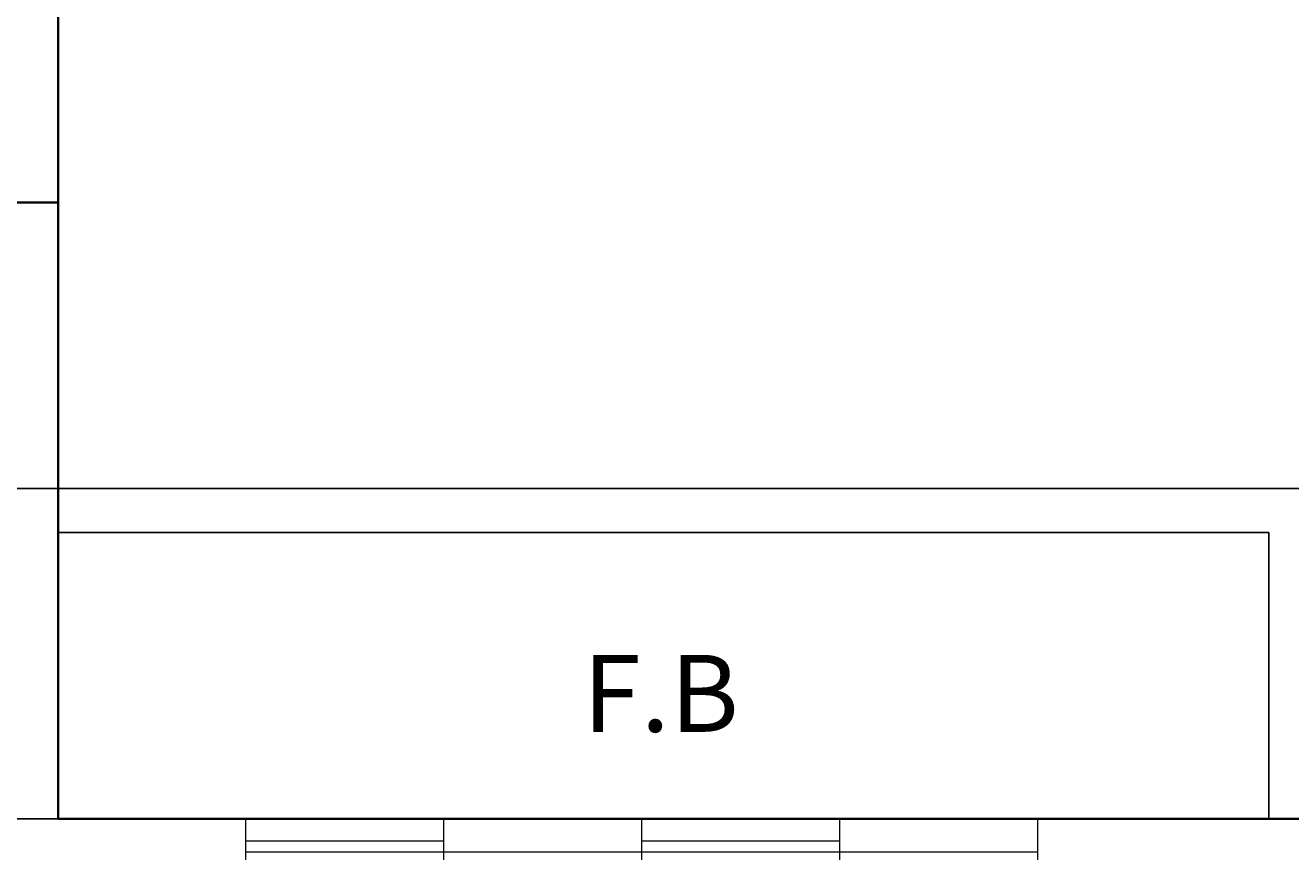
# Model space of a CAD drawing. Units: feet. Extents: x 105 to 1094, y -88 to 588.
# Tile 41 of 59: x 436 to 551, y 438 to 513. Entities that reach past the tile are written whole.
import ezdxf

# ---------------------------------------------------------------- set-up
doc = ezdxf.new("R2010")
doc.units = ezdxf.units.FT
doc.header["$MEASUREMENT"] = 0
for name, color, linetype, lineweight in [('A-ANNO-DIMS', 2, 'Continuous', 18), ('A-ANNO-TEXT', 7, 'Continuous', 18), ('A-FLOR-PROJ', 8, 'Continuous', 25), ('A-GLAZ', 4, 'Continuous', 18), ('A-WALL', 7, 'Continuous', 35)]:
    doc.layers.add(name, color=color, linetype=linetype, lineweight=lineweight)
doc.styles.get("Standard").update_dxf_attribs({"font": 'arial.ttf'})
doc.dimstyles.get("Standard").update_dxf_attribs({"dimtxt": 0.18, "dimasz": 0.18, "dimexe": 0.18, "dimexo": 0.0625, "dimgap": 0.09, "dimtad": 0, "dimtih": 1, "dimtoh": 1, "dimdec": 4, "dimzin": 0, "dimdsep": 46, "dimtxsty": 'Standard', "dimcen": 0.09, "dimadec": 0, "dimazin": 0, "dimtfac": 1, "dimtdec": 4, "dimtofl": 0, "dimtmove": 0, "dimatfit": 3, "dimfxl": 1, "dimtolj": 1, "dimtzin": 0, "dimarcsym": 0})

# ---------------------------------------------------------------- blocks, each defined once
blk = doc.blocks.new('WIN-FOUR-LIGHT-WIDE')
for p, q in [((0, 0), (0, 6)), ((18, 0), (18, 6)), ((36, 0), (36, 6)), ((54, 0), (54, 6)), ((72, 0), (72, 6)), ((18, 4), (36, 4)), ((54, 4), (72, 4)), ((0, 3), (72, 3)), ((0, 2), (18, 2)), ((36, 2), (54, 2))]:
    blk.add_line(p, q)
blk = doc.blocks.new('*D21')
at = {"layer": 'A-ANNO-DIMS', "color": 0, "lineweight": -2, "transparency": 16777216}
for p, q in [((849.63, 543.08), (105.46, 543.08)), ((105.64, 542.9), (105.64, 250.26)), ((105.64, -42.74), (105.64, 249.9)), ((849.63, -42.92), (105.46, -42.92))]:
    blk.add_line(p, q, dxfattribs=at)
at = {"layer": 'A-ANNO-DIMS', "color": 0, "transparency": 16777216}
for points in [[(105.61, 542.9), (105.67, 542.9), (105.64, 543.08)], [(105.61, -42.74), (105.67, -42.74), (105.64, -42.92)]]:
    blk.add_solid(points, dxfattribs=at)
at = {"layer": 'Defpoints', "color": 0, "transparency": 16777216}
for p in [(105.64, 543.08), (849.69, 543.08), (849.69, -42.92)]:
    blk.add_point(p, dxfattribs=at)
at = {"layer": 'A-ANNO-DIMS', "color": 0, "transparency": 16777216, "insert": (105.64, 250.08), "char_height": 0.18, "attachment_point": 5}
blk.add_mtext('\\A1;586', dxfattribs=at)
blk = doc.blocks.new('*D25')
at = {"layer": 'A-ANNO-DIMS', "color": 0, "lineweight": -2, "transparency": 16777216}
for p, q in [((438.69, 527.14), (438.69, 588.31)), ((438.87, 588.13), (495.41, 588.13)), ((552.51, 588.13), (495.97, 588.13)), ((552.69, 471.14), (552.69, 588.31))]:
    blk.add_line(p, q, dxfattribs=at)
at = {"layer": 'A-ANNO-DIMS', "color": 0, "transparency": 16777216}
for points in [[(438.87, 588.16), (438.87, 588.1), (438.69, 588.13)], [(552.51, 588.16), (552.51, 588.1), (552.69, 588.13)]]:
    blk.add_solid(points, dxfattribs=at)
at = {"layer": 'Defpoints', "color": 0, "transparency": 16777216}
for p in [(552.69, 588.13), (438.69, 527.08), (552.69, 471.08)]:
    blk.add_point(p, dxfattribs=at)
at = {"layer": 'A-ANNO-DIMS', "color": 0, "transparency": 16777216, "insert": (495.69, 588.13), "char_height": 0.18, "attachment_point": 5}
blk.add_mtext('\\A1;114', dxfattribs=at)
blk = doc.blocks.new('*D31')
at = {"layer": 'A-ANNO-DIMS', "color": 0, "lineweight": -2, "transparency": 16777216}
for p, q in [((438.75, 527.08), (1093.92, 527.08)), ((1093.74, 526.9), (1093.74, 499.26)), ((1093.74, 471.26), (1093.74, 498.9)), ((438.75, 471.08), (1093.92, 471.08))]:
    blk.add_line(p, q, dxfattribs=at)
at = {"layer": 'A-ANNO-DIMS', "color": 0, "transparency": 16777216}
for points in [[(1093.71, 526.9), (1093.77, 526.9), (1093.74, 527.08)], [(1093.71, 471.26), (1093.77, 471.26), (1093.74, 471.08)]]:
    blk.add_solid(points, dxfattribs=at)
at = {"layer": 'Defpoints', "color": 0, "transparency": 16777216}
for p in [(438.69, 527.08), (1093.74, 527.08), (438.69, 471.08)]:
    blk.add_point(p, dxfattribs=at)
at = {"layer": 'A-ANNO-DIMS', "color": 0, "transparency": 16777216, "insert": (1093.74, 499.08), "char_height": 0.18, "attachment_point": 5}
blk.add_mtext('\\A1;56', dxfattribs=at)
blk = doc.blocks.new('*D32')
at = {"layer": 'A-ANNO-DIMS', "color": 0, "lineweight": -2, "transparency": 16777216}
for p, q in [((646.63, 471.08), (105.46, 471.08)), ((105.64, 470.9), (105.64, 456.26)), ((105.64, 441.26), (105.64, 455.9)), ((646.63, 441.08), (105.46, 441.08))]:
    blk.add_line(p, q, dxfattribs=at)
at = {"layer": 'A-ANNO-DIMS', "color": 0, "transparency": 16777216}
for points in [[(105.61, 470.9), (105.67, 470.9), (105.64, 471.08)], [(105.61, 441.26), (105.67, 441.26), (105.64, 441.08)]]:
    blk.add_solid(points, dxfattribs=at)
at = {"layer": 'Defpoints', "color": 0, "transparency": 16777216}
for p in [(105.64, 471.08), (646.69, 471.08), (646.69, 441.08)]:
    blk.add_point(p, dxfattribs=at)
at = {"layer": 'A-ANNO-DIMS', "color": 0, "transparency": 16777216, "insert": (105.64, 456.08), "char_height": 0.18, "attachment_point": 5}
blk.add_mtext('\\A1;30', dxfattribs=at)

msp = doc.modelspace()

# ---------------------------------------------------------------- linework, layer by layer
at = {"layer": 'A-FLOR-PROJ'}
for p, q in [((438.6883, 471.0812), (552.6883, 471.0812)), ((438.6883, 467.0812), (548.6883, 467.0812)), ((548.6883, 467.0812), (548.6883, 441.0812))]:
    msp.add_line(p, q, dxfattribs=at)
at = {"layer": 'A-WALL'}
for p, q in [((438.6883, 527.0812), (438.6883, 441.0812)), ((438.6883, 497.0812), (349.6883, 497.0812)), ((438.6883, 441.0812), (552.6883, 441.0812))]:
    msp.add_line(p, q, dxfattribs=at)

# ---------------------------------------------------------------- block references
at = {"layer": 'A-GLAZ', "extrusion": (0, 0, -1), "zscale": -1, "rotation": 180}
msp.add_blockref('WIN-FOUR-LIGHT-WIDE', (-455.688, 441.0813), dxfattribs=at)

# ---------------------------------------------------------------- texts
at = {"layer": 'A-ANNO-TEXT', "insert": (542.6156, 455.9748), "char_height": 7, "attachment_point": 3}
msp.add_mtext_dynamic_manual_height_columns('\\pxqc;F.B ', width=98.34246, gutter_width=1, heights=[0], dxfattribs=at)

# ---------------------------------------------------------------- dimensions: what is measured, and where the dimension line sits
at = {"layer": 'A-ANNO-DIMS'}
dim = msp.add_linear_dim(base=(552.6883, 588.1312), p1=(438.6883, 527.0812), p2=(552.6883, 471.0812), dimstyle='Standard', override={"dimdec": 0, "dimlfac": 1, "dimrnd": 0, "dimzin": 0, "dimdsep": 46, "dimlunit": 2}, dxfattribs=at)
dim.commit()
dim.dimension.update_dxf_attribs({"geometry": '*D25', "text_midpoint": (495.6883, 588.1312)})
for base, p1, p2, picture, middle in [((105.6383, 543.0812), (849.6883, -42.9188), (849.6883, 543.0812), '*D21', (105.6383, 250.0812)), ((1093.7383, 527.0812), (438.6883, 471.0812), (438.6883, 527.0812), '*D31', (1093.7383, 499.0812)), ((105.6383, 471.0812), (646.6883, 441.0812), (646.6883, 471.0812), '*D32', (105.6383, 456.0812))]:
    dim = msp.add_linear_dim(base=base, p1=p1, p2=p2, angle=90, dimstyle='Standard', override={"dimdec": 0, "dimlfac": 1, "dimrnd": 0, "dimzin": 0, "dimdsep": 46, "dimlunit": 2}, dxfattribs=at)
    dim.commit()
    dim.dimension.update_dxf_attribs({"geometry": picture, "text_midpoint": middle})

doc.saveas('drawing.dxf')
